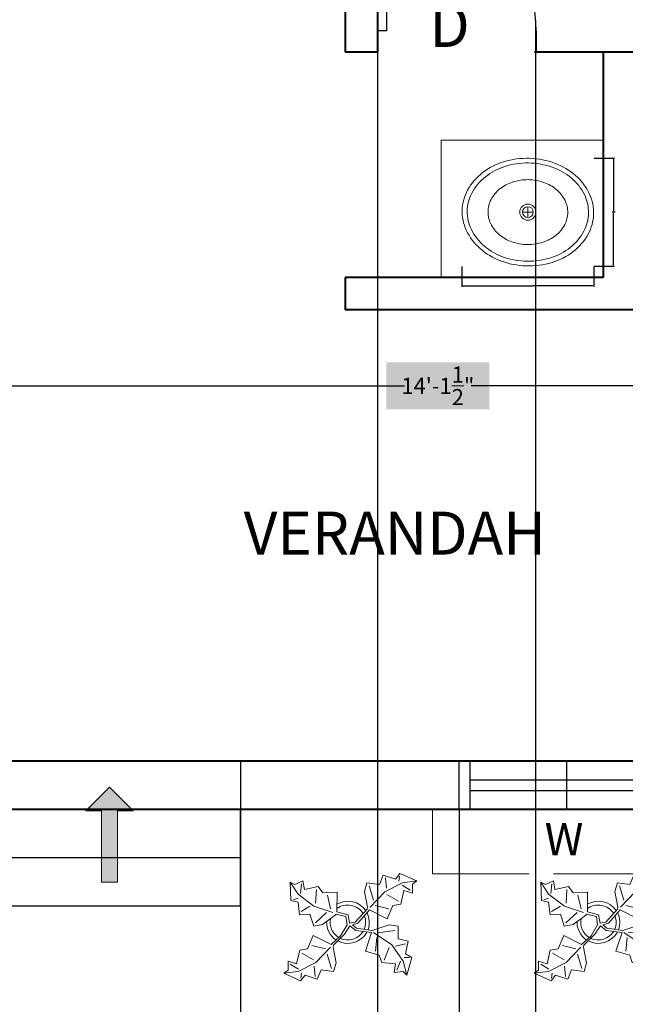
# Model space of a CAD drawing. Units: inches. Extents: x -301 to 715, y -607 to 364.
# Tile 86 of 141: x -39 to 74, y -260 to -77. Entities that reach past the tile are written whole.
import ezdxf

# ---------------------------------------------------------------- set-up
doc = ezdxf.new("R2010")
doc.units = ezdxf.units.IN
doc.header["$MEASUREMENT"] = 0
doc.linetypes.add('ACAD_ISO02W100', pattern=[15, 12, -3])
for name, color, linetype, lineweight in [('A-ANNO-DIMS', 2, 'Continuous', 18), ('A-ANNO-SYMB', 4, 'Continuous', 18), ('A-ANNO-TEXT', 4, 'Continuous', 18), ('A-AREA-IDEN', 220, 'Continuous', 25), ('A-DOOR', 4, 'Continuous', 25), ('A-FLOR-CASE', 8, 'Continuous', 18), ('A-FLOR-FIXT', 9, 'Continuous', 18), ('A-FLOR-STRS', 2, 'Continuous', 25), ('A-GLAZ', 2, 'Continuous', 25), ('A-GLAZ-OVHD', 2, 'ACAD_ISO02W100', 18), ('A-WALL', 3, 'Continuous', 40), ('L-PLNT', 94, 'Continuous', 13)]:
    doc.layers.add(name, color=color, linetype=linetype, lineweight=lineweight)
doc.styles.get("Standard").update_dxf_attribs({"font": 'arial.ttf'})
doc.dimstyles.get("Standard").update_dxf_attribs({"dimtxt": 0.18, "dimasz": 0.18, "dimexe": 0.18, "dimexo": 0.0625, "dimgap": 0.09, "dimtad": 0, "dimtih": 1, "dimtoh": 1, "dimdec": 1, "dimzin": 0, "dimdsep": 46, "dimlunit": 4, "dimtxsty": 'Standard', "dimcen": 0.09, "dimclrd": 3, "dimclre": 4, "dimclrt": 6, "dimadec": 0, "dimazin": 0, "dimtfac": 1, "dimtdec": 1, "dimtofl": 0, "dimtmove": 0, "dimatfit": 3, "dimfxl": 1, "dimtfill": 2, "dimtfillclr": 51, "dimtolj": 1, "dimtzin": 0, "dimarcsym": 0})

# ---------------------------------------------------------------- blocks, each defined once
blk = doc.blocks.new('*U2')
for p, q in [((0, 0), (0, -100)), ((750, 0), (750, -100))]:
    blk.add_line(p, q)
blk.add_lwpolyline([(0, 0), (0, 750), (43.75, 750), (43.75, 0)], close=True)
blk.add_arc((0, 0), 750, 0, 90)
blk = doc.blocks.new('Sink - Oval top')
for p, q in [((-1, 0), (1, 0)), ((0, 1), (0, -1))]:
    blk.add_line(p, q)
for points in [[(-12.23, 0.39, 0.117634), (-11.46, -3.36, 0.104469), (-8.88, -6.8, 0.090016), (-5.08, -9.07, 0.08192), (-0.32, -10.02, 0.08192), (4.49, -9.38, 0.090016), (8.42, -7.36, 0.104469), (11.22, -4.09, 0.117634), (12.23, -0.39, 0.117634), (11.46, 3.36, 0.104469), (8.88, 6.8, 0.090016), (5.08, 9.07, 0.08192), (0.32, 10.02, 0.08192), (-4.49, 9.38, 0.090016), (-8.42, 7.36, 0.104469), (-11.22, 4.09, 0.117634)], [(-11.29, 0.16, 0.118622), (-10.52, -3.25, 0.104678), (-8.07, -6.36, 0.089562), (-4.54, -8.37, 0.081185), (-0.13, -9.15, 0.081185), (4.3, -8.49, 0.089562), (7.89, -6.58, 0.104678), (10.42, -3.55, 0.118622), (11.29, -0.16, 0.118622), (10.52, 3.25, 0.104678), (8.07, 6.36, 0.089562), (4.54, 8.37, 0.081185), (0.13, 9.15, 0.081185), (-4.3, 8.49, 0.089562), (-7.89, 6.58, 0.104678), (-10.42, 3.55, 0.118622)], [(-7.42, 0.08, 0.118283), (-6.91, -2.17, 0.104607), (-5.29, -4.21, 0.089718), (-2.97, -5.53, 0.081436), (-0.07, -6.04, 0.081436), (2.84, -5.59, 0.089718), (5.2, -4.33, 0.104607), (6.86, -2.32, 0.118283), (7.42, -0.08, 0.118283), (6.91, 2.17, 0.104607), (5.29, 4.21, 0.089718), (2.97, 5.53, 0.081436), (0.07, 6.04, 0.081436), (-2.84, 5.59, 0.089718), (-5.2, 4.33, 0.104607), (-6.86, 2.32, 0.118283)]]:
    blk.add_lwpolyline(points, format="xyb", close=True)
for radius in [1.5, 1]:
    blk.add_circle((0, 0), radius)
blk = doc.blocks.new('Plant - Rubber or Philodendron')
for p, q in [((13.3837, 12.301), (14.68, 13.9039)), ((14.68, 13.9039), (19.3848, 11.8146)), ((-16.2005, 11.4774), (-13.9899, 8.1064)), ((-16.2005, 11.4774), (-14.8639, 10.7964)), ((-16.0159, 6.3329), (-16.2005, 11.4774)), ((-14.8639, 10.7964), (-12.6195, 11.8975)), ((-12.6195, 11.8975), (-12.1909, 9.4345)), ((4.6914, 8.8812), (5.3859, 11.2828)), ((5.3859, 11.2828), (8.8871, 10.7908)), ((8.8871, 10.7908), (9.9809, 13.4933)), ((9.9809, 13.4933), (13.3837, 12.301)), ((15.3859, 11.3055), (10.3916, 8.7942)), ((10.5828, 12.6946), (10.8893, 9.7953)), ((14.5816, 13.2037), (14.3848, 11.8033)), ((19.3848, 11.8146), (15.3859, 11.3055)), ((19.3848, 11.8146), (18.1868, 10.9119)), ((-13.3174, 8.325), (-13.0735, 11.0065)), ((-12.1909, 9.4345), (-8.3829, 10.3)), ((-8.8369, 9.409), (-9.0894, 5.6095)), ((-8.3829, 10.3), (-7.0549, 8.501)), ((-7.0549, 8.501), (-3.0284, 8.6941)), ((-3.0284, 8.6941), (-3.0709, 3.1041)), ((4.6914, 8.8812), (5.5014, 4.4831)), ((5.9878, 10.4842), (7.1971, 6.3869)), ((10.3916, 8.7942), (6.2847, 4.4028)), ((15.7909, 9.1065), (14.8995, 5.3044)), ((15.2875, 10.6053), (17.5907, 9.2105)), ((18.1925, 8.4119), (15.7909, 9.1065)), ((18.1868, 10.9119), (18.1925, 8.4119)), ((-14.0069, 5.8704), (-16.0159, 6.3329)), ((-15.3434, 6.5514), (-13.9984, 6.9884)), ((-13.5868, 2.2894), (-14.0069, 5.8704)), ((-13.9899, 8.1064), (-9.5434, 4.7185)), ((-4.8529, 4.012), (-5.7184, 7.82)), ((14.2977, 6.1031), (10.9934, 7.9956)), ((-13.1329, 3.1804), (-10.6614, 4.727)), ((-9.5434, 4.7185), (-4.1917, 2.9888)), ((-9.1318, 0.0195), (-5.9793, 2.9025)), ((-3.0709, 3.1041), (0.0797, 2.3163)), ((2.1141, 0.2298), (5.4346, 3.9146)), ((6.1032, 3.6844), (2.8262, -0.031)), ((5.4346, 3.9146), (5.5014, 4.4831)), ((11.1089, 1.1958), (6.1032, 3.6844)), ((7.7005, 4.8881), (11.5025, 3.9967)), ((12.7005, 4.8994), (11.1089, 1.1958)), ((14.8995, 5.3044), (12.7005, 4.8994)), ((-10.6784, 2.491), (-13.5868, 2.2894)), ((-9.5858, -0.8715), (-10.6784, 2.491)), ((-7.1228, -0.443), (-3.5248, 2.2131)), ((-3.5248, 2.2131), (-3.3011, 2.4355)), ((-3.3011, 2.4355), (-0.5306, 1.7947)), ((-0.5306, 1.7947), (-0.2255, -0.5527)), ((-0.5306, 1.7947), (-0.5306, 1.7947)), ((0.0797, 2.3163), (0.4866, -0.031)), ((0.4866, -0.031), (2.1141, 0.2298)), ((-7.1228, -0.443), (-9.5858, -0.8715)), ((-2.019, -3.6148), (-0.2255, -0.5527)), ((-0.9375, -3.1608), (0.5883, -0.8135)), ((0.5883, -0.8135), (2.2447, -2.0916)), ((2.8262, -0.031), (1.3003, -0.5527)), ((1.3003, -0.5527), (2.4193, -1.4655)), ((2.2447, -2.0916), (6.7108, -2.6626)), ((2.4193, -1.4655), (6.895, -2.1175)), ((4.943, -7.9659), (6.7108, -2.6626)), ((11.6605, -0.5413), (6.895, -2.1175)), ((12.3677, -6.1981), (7.219, -2.6772)), ((8.3544, -2.7453), (13.1973, -2.1704)), ((11.6605, -0.5413), (14.1354, -0.8948)), ((14.1354, -0.8948), (14.1354, -4.4304)), ((-11.3237, -7.2629), (-9.7321, -3.5593)), ((-9.7321, -3.5593), (-4.7264, -6.0479)), ((-2.019, -3.6148), (-4.7264, -6.0479)), ((-4.0579, -6.2781), (-0.9375, -3.1608)), ((8.125, -4.0768), (7.7715, -7.9659)), ((14.1354, -4.4304), (16.9638, -5.1375)), ((16.9638, -5.1375), (16.2567, -8.673)), ((-14.4141, -11.4699), (-13.5228, -7.6679)), ((-13.5228, -7.6679), (-11.3237, -7.2629)), ((-6.3237, -7.2516), (-10.1257, -6.3602)), ((-9.0148, -11.1577), (-4.9047, -6.8122)), ((-4.1246, -6.8466), (-4.0579, -6.2781)), ((-3.3146, -11.2447), (-4.1246, -6.8466)), ((8.8321, -9.0266), (4.943, -7.9659)), ((10.2463, -10.4408), (11.6605, -6.9053)), ((15.5496, -10.7943), (12.3677, -6.1981)), ((16.2567, -5.8446), (13.4283, -6.5517)), ((-16.8157, -10.7754), (-14.4141, -11.4699)), ((-16.8101, -13.2754), (-16.8157, -10.7754)), ((-12.921, -8.4665), (-9.6166, -10.359)), ((-4.611, -12.8477), (-5.8203, -8.7504)), ((9.5392, -11.1479), (8.8321, -9.0266)), ((14.8425, -10.7943), (13.7819, -13.2692)), ((16.6103, -14.6834), (15.5496, -10.7943)), ((17.3174, -9.7337), (15.9032, -9.7337)), ((16.2567, -8.673), (18.0245, -9.7337)), ((18.0245, -9.7337), (16.6103, -14.6834)), ((-18.008, -14.1781), (-16.8101, -13.2754)), ((-18.008, -14.1781), (-14.0091, -13.669)), ((-13.9107, -12.9688), (-16.2139, -11.574)), ((-14.0091, -13.669), (-9.0148, -11.1577)), ((-9.206, -15.0581), (-9.5126, -12.1588)), ((-7.5103, -13.1543), (-8.6042, -15.8568)), ((-4.0092, -13.6463), (-7.5103, -13.1543)), ((-3.3146, -11.2447), (-4.0092, -13.6463)), ((13.4283, -11.5015), (9.5392, -11.1479)), ((13.0748, -13.9763), (13.4283, -11.5015)), ((15.5496, -13.6228), (13.0748, -13.9763)), ((16.6103, -14.6834), (15.5496, -13.6228)), ((-13.3032, -16.2674), (-18.008, -14.1781)), ((-12.0069, -14.6645), (-13.3032, -16.2674)), ((-13.2048, -15.5672), (-13.008, -14.1668)), ((-8.6042, -15.8568), (-12.0069, -14.6645))]:
    blk.add_line(p, q)
for centre, radius, start, end in [((0, 0), 6.1275, 34.37569, 120.1028), ((-0.0601, -0.2075), 5.2461, 33.82192, 124.9414), ((-0.098, 0.1364), 6.1288, 341.2017, 26.09184), ((0.0308, 0.1664), 6, 178.6147, 235.1169), ((0.0308, 0.1664), 5, 168.1647, 238.6725), ((-0.2664, 0.1682), 5.2775, 338.4094, 20.03007), ((-0.0234, 0.3825), 6.1492, 242.5812, 331.2714), ((-0.1102, 0.4886), 5.2883, 247.3711, 327.472)]:
    blk.add_arc(centre, radius, start, end)
blk = doc.blocks.new('*U28')
h = blk.add_hatch(color=0)
h.set_gradient(color1=(0, 0, 255), rotation=180, tint=1)
h.paths.add_polyline_path([(0, 0), (-0.25, -0.25), (-0.25, -0.085), (-1, -0.085), (-1, 0.085), (-0.25, 0.085), (-0.25, 0.25)])
at = {"color": 0}
blk.add_lwpolyline([(0, 0), (-0.25, -0.25), (-0.25, -0.085), (-1, -0.085), (-1, 0.085), (-0.25, 0.085), (-0.25, 0.25)], close=True, dxfattribs=at)
blk = doc.blocks.new('*D42')
at = {"layer": 'A-ANNO-DIMS', "color": 0, "lineweight": -2, "transparency": 16777216}
for p, q in [((-45.6, -130.88), (-45.6, -145.16)), ((123.9, -130.88), (123.9, -145.16)), ((-40.6, -144.98), (32.95, -144.98)), ((118.9, -144.98), (45.34, -144.98))]:
    blk.add_line(p, q, dxfattribs=at)
at = {"layer": 'A-ANNO-DIMS', "color": 0, "transparency": 16777216}
for points in [[(-40.6, -144.15), (-40.6, -145.82), (-45.6, -144.98)], [(118.9, -144.15), (118.9, -145.82), (123.9, -144.98)]]:
    blk.add_solid(points, dxfattribs=at)
at = {"layer": 'Defpoints', "color": 0, "transparency": 16777216}
for p in [(-45.6, -130.82), (123.9, -130.82), (-45.6, -144.98)]:
    blk.add_point(p, dxfattribs=at)
at = {"layer": 'A-ANNO-DIMS', "color": 0, "transparency": 16777216, "insert": (39.15, -144.98), "char_height": 3, "attachment_point": 5, "bg_fill": 1, "box_fill_scale": 1.25, "bg_fill_color": 51, "bg_fill_transparency": 0}
blk.add_mtext('\\A1;14\'-1{\\H1x;\\S1/2;}"', dxfattribs=at)
blk = doc.blocks.new('WIN-36-PLAN')
for p, q in [((0, 0), (0, 9)), ((2, 0), (2, 9)), ((20, 0), (20, 9)), ((38, 0), (38, 9)), ((40, 0), (40, 9)), ((2, 5.5), (38, 5.5)), ((2, 3.5), (38, 3.5))]:
    blk.add_line(p, q)
blk = doc.blocks.new('WIN-SHADE-50')
at = {"ltscale": 1.5}
for p, q in [((0, 0), (0, 12)), ((50, 12), (0, 12)), ((50, 0), (50, 12)), ((5, 0), (0, 0)), ((45, 0), (50, 0))]:
    blk.add_line(p, q, dxfattribs=at)
blk = doc.blocks.new('ENTRY-STEPS-48')
for p, q in [((0, 27), (0, 18)), ((48, 27), (48, 18)), ((0, 18), (0, 9)), ((48, 9), (48, 18)), ((0, 9), (48, 9)), ((0, 9), (0, 0)), ((48, 0), (48, 9)), ((0, 0), (48, 0))]:
    blk.add_line(p, q)
blk = doc.blocks.new('*D126')
at = {"layer": 'A-ANNO-DIMS', "color": 4, "lineweight": -2, "transparency": 16777216}
for p, q in [((43.63, -122.77), (43.63, -126.57)), ((68.18, -122.77), (68.18, -126.57))]:
    blk.add_line(p, q, dxfattribs=at)
at = {"layer": 'A-ANNO-DIMS', "color": 3, "lineweight": -2, "transparency": 16777216}
for p, q in [((43.81, -126.39), (54.96, -126.39)), ((68, -126.39), (56.85, -126.39))]:
    blk.add_line(p, q, dxfattribs=at)
at = {"layer": 'A-ANNO-DIMS', "color": 3, "transparency": 16777216}
for points in [[(43.81, -126.36), (43.81, -126.42), (43.63, -126.39)], [(68, -126.36), (68, -126.42), (68.18, -126.39)]]:
    blk.add_solid(points, dxfattribs=at)
at = {"layer": 'Defpoints', "color": 0, "transparency": 16777216}
for p in [(43.63, -122.71), (68.18, -122.71), (68.18, -126.39)]:
    blk.add_point(p, dxfattribs=at)
at = {"layer": 'A-ANNO-DIMS', "color": 6, "transparency": 16777216, "insert": (55.91, -126.39), "char_height": 0.18, "attachment_point": 5, "bg_fill": 1, "box_fill_scale": 1.25, "bg_fill_color": 51, "bg_fill_transparency": 0}
blk.add_mtext('\\A1;BASIN 2\'-0 1/2"', dxfattribs=at)
blk = doc.blocks.new('*D127')
at = {"layer": 'A-ANNO-DIMS', "color": 4, "lineweight": -2, "transparency": 16777216}
for p, q in [((68.25, -102.57), (72.05, -102.57)), ((68.25, -122.71), (72.05, -122.71))]:
    blk.add_line(p, q, dxfattribs=at)
at = {"layer": 'A-ANNO-DIMS', "color": 3, "lineweight": -2, "transparency": 16777216}
for p, q in [((71.87, -102.75), (71.87, -112.46)), ((71.87, -122.53), (71.87, -112.82))]:
    blk.add_line(p, q, dxfattribs=at)
at = {"layer": 'A-ANNO-DIMS', "color": 3, "transparency": 16777216}
for points in [[(71.84, -102.75), (71.9, -102.75), (71.87, -102.57)], [(71.84, -122.53), (71.9, -122.53), (71.87, -122.71)]]:
    blk.add_solid(points, dxfattribs=at)
at = {"layer": 'Defpoints', "color": 0, "transparency": 16777216}
for p in [(68.18, -102.57), (71.87, -102.57), (68.18, -122.71)]:
    blk.add_point(p, dxfattribs=at)
at = {"layer": 'A-ANNO-DIMS', "color": 6, "transparency": 16777216, "insert": (71.87, -112.64), "char_height": 0.18, "attachment_point": 5, "bg_fill": 1, "box_fill_scale": 1.25, "bg_fill_color": 51, "bg_fill_transparency": 0}
blk.add_mtext('\\A1;1\'-8"', dxfattribs=at)
blk = doc.blocks.new('*D148')
at = {"layer": 'A-ANNO-DIMS', "color": 4, "lineweight": -2, "transparency": 16777216}
for p, q in [((2.4, -223.88), (2.4, -296.87)), ((43.15, -223.88), (43.15, -296.87))]:
    blk.add_line(p, q, dxfattribs=at)
at = {"layer": 'A-ANNO-DIMS', "color": 3, "lineweight": -2, "transparency": 16777216}
for p, q in [((2.58, -296.69), (22.44, -296.69)), ((42.97, -296.69), (23.1, -296.69))]:
    blk.add_line(p, q, dxfattribs=at)
at = {"layer": 'A-ANNO-DIMS', "color": 3, "transparency": 16777216}
for points in [[(2.58, -296.66), (2.58, -296.72), (2.4, -296.69)], [(42.97, -296.66), (42.97, -296.72), (43.15, -296.69)]]:
    blk.add_solid(points, dxfattribs=at)
at = {"layer": 'Defpoints', "color": 0, "transparency": 16777216}
for p in [(2.4, -223.82), (43.15, -223.82), (43.15, -296.69)]:
    blk.add_point(p, dxfattribs=at)
at = {"layer": 'A-ANNO-DIMS', "color": 6, "transparency": 16777216, "insert": (22.77, -296.69), "char_height": 0.18, "attachment_point": 5, "bg_fill": 1, "box_fill_scale": 1.25, "bg_fill_color": 51, "bg_fill_transparency": 0}
blk.add_mtext('\\A1;3\'-5"', dxfattribs=at)
blk = doc.blocks.new('*D160')
at = {"layer": 'A-ANNO-DIMS', "color": 4, "lineweight": -2, "transparency": 16777216}
for p, q in [((57.35, -76.88), (57.35, -296.87)), ((27.9, -78.94), (27.9, -296.87))]:
    blk.add_line(p, q, dxfattribs=at)
at = {"layer": 'A-ANNO-DIMS', "color": 3, "lineweight": -2, "transparency": 16777216}
for p, q in [((28.08, -296.69), (42.08, -296.69)), ((57.17, -296.69), (43.16, -296.69))]:
    blk.add_line(p, q, dxfattribs=at)
at = {"layer": 'A-ANNO-DIMS', "color": 3, "transparency": 16777216}
for points in [[(28.08, -296.66), (28.08, -296.72), (27.9, -296.69)], [(57.17, -296.66), (57.17, -296.72), (57.35, -296.69)]]:
    blk.add_solid(points, dxfattribs=at)
at = {"layer": 'Defpoints', "color": 0, "transparency": 16777216}
for p in [(57.35, -76.82), (27.9, -78.88), (57.35, -296.69)]:
    blk.add_point(p, dxfattribs=at)
at = {"layer": 'A-ANNO-DIMS', "color": 6, "transparency": 16777216, "insert": (42.62, -296.69), "char_height": 0.18, "attachment_point": 5, "bg_fill": 1, "box_fill_scale": 1.25, "bg_fill_color": 51, "bg_fill_transparency": 0}
blk.add_mtext('\\A1;2\'-5 1/2"', dxfattribs=at)

msp = doc.modelspace()

# ---------------------------------------------------------------- linework, layer by layer
at = {"layer": 'A-FLOR-CASE'}
for q in [(69.9, -99.23), (39.79, -124.82)]:
    msp.add_line((39.79, -99.23), q, dxfattribs=at)
at = {"layer": 'A-WALL'}
for p, q in [((21.9, -9.82), (21.9, -82.82)), ((27.9, -15.82), (27.9, -82.82)), ((21.9, -82.82), (27.9, -82.82)), ((57.16, -82.82), (123.9, -82.82)), ((69.9, -82.82), (69.9, -124.82)), ((69.9, -124.82), (21.9, -124.82)), ((21.9, -124.82), (21.9, -130.82)), ((75.9, -130.82), (21.9, -130.82)), ((-45.84, -214.82), (123.9, -214.82)), ((-45.6, -223.82), (132.9, -223.82))]:
    msp.add_line(p, q, dxfattribs=at)

# ---------------------------------------------------------------- block references
at = {"layer": 'A-ANNO-SYMB', "xscale": 17.68611049110349, "yscale": 17.68611049110349, "zscale": 17.68611049110349, "rotation": 90}
msp.add_blockref('*U28', (-21.96, -219.71), dxfattribs=at)
at = {"layer": 'A-DOOR', "xscale": 0.0393700787401575, "yscale": 0.0393700787401575, "zscale": 0.0393700787401575}
msp.add_blockref('*U2', (27.9, -78.88), dxfattribs=at)
at = {"layer": 'A-FLOR-FIXT'}
msp.add_blockref('Sink - Oval top', (55.91, -112.64), dxfattribs=at)
at = {"layer": 'A-FLOR-STRS'}
msp.add_blockref('ENTRY-STEPS-48', (-45.6, -241.82), dxfattribs=at)
at = {"layer": 'A-GLAZ'}
msp.add_blockref('WIN-36-PLAN', (43.15, -223.82), dxfattribs=at)
at = {"layer": 'A-GLAZ-OVHD', "rotation": 180}
msp.add_blockref('WIN-SHADE-50', (88.15, -223.82), dxfattribs=at)
at = {"layer": 'L-PLNT', "xscale": 0.6613521884636907, "yscale": 0.6613521884636907, "zscale": 0.6613521884636907}
for p in [(22.4, -244.98), (69.02, -244.98)]:
    msp.add_blockref('Plant - Rubber or Philodendron', p, dxfattribs=at)

# ---------------------------------------------------------------- texts
at = {"layer": 'A-ANNO-TEXT'}
for s, height, p in [('D', 8, (37.58, -81.89)), ('W', 6, (59.04, -232.4))]:
    msp.add_text(s, height=height, dxfattribs=at).set_placement(p)
at = {"layer": 'A-AREA-IDEN', "insert": (3.02, -168.41), "char_height": 8, "attachment_point": 1}
msp.add_mtext_dynamic_manual_height_columns('VERANDAH', width=73.06, gutter_width=1, heights=[0], dxfattribs=at)

# ---------------------------------------------------------------- dimensions: what is measured, and where the dimension line sits
at = {"layer": 'A-ANNO-DIMS'}
for base, p1, p2, override, picture, middle in [((57.3521, -296.6855), (27.8967, -78.8807), (57.3521, -76.8177), {"dimdec": 1, "dimlfac": 1, "dimrnd": 0, "dimzin": 1, "dimdsep": 46, "dimlunit": 4, "dimfrac": 2}, '*D160', (42.6244, -296.6855)), ((-45.6, -144.98), (123.9, -130.82), (-45.6, -130.82), {"dimtxt": 3, "dimasz": 5, "dimclrd": 0, "dimclre": 0, "dimclrt": 0}, '*D42', (39.15, -144.98)), ((43.146712, -296.685468), (2.396712, -223.81767), (43.146712, -223.81767), {"dimdec": 1, "dimlfac": 1, "dimrnd": 0, "dimzin": 1, "dimdsep": 46, "dimlunit": 4, "dimfrac": 2}, '*D148', (22.771712, -296.685468))]:
    dim = msp.add_linear_dim(base=base, p1=p1, p2=p2, dimstyle='Standard', override=override, dxfattribs=at)
    dim.commit()
    dim.dimension.update_dxf_attribs({"geometry": picture, "text_midpoint": middle})
dim = msp.add_linear_dim(base=(71.87, -102.57), p1=(68.18, -122.71), p2=(68.18, -102.57), angle=90, dimstyle='Standard', override={"dimdec": 1, "dimlfac": 1, "dimrnd": 0, "dimzin": 1, "dimdsep": 46, "dimlunit": 4, "dimfrac": 2}, dxfattribs=at)
dim.commit()
dim.dimension.update_dxf_attribs({"geometry": '*D127', "text_midpoint": (71.87, -112.64)})
dim = msp.add_linear_dim(base=(68.1827, -126.3927), p1=(43.6319, -122.71), p2=(68.1827, -122.71), text='BASIN <>', dimstyle='Standard', override={"dimdec": 1, "dimlfac": 1, "dimrnd": 0, "dimzin": 1, "dimdsep": 46, "dimlunit": 4, "dimfrac": 2}, dxfattribs=at)
dim.commit()
dim.dimension.update_dxf_attribs({"geometry": '*D126', "text_midpoint": (55.9073, -126.3927)})

doc.saveas('drawing.dxf')
